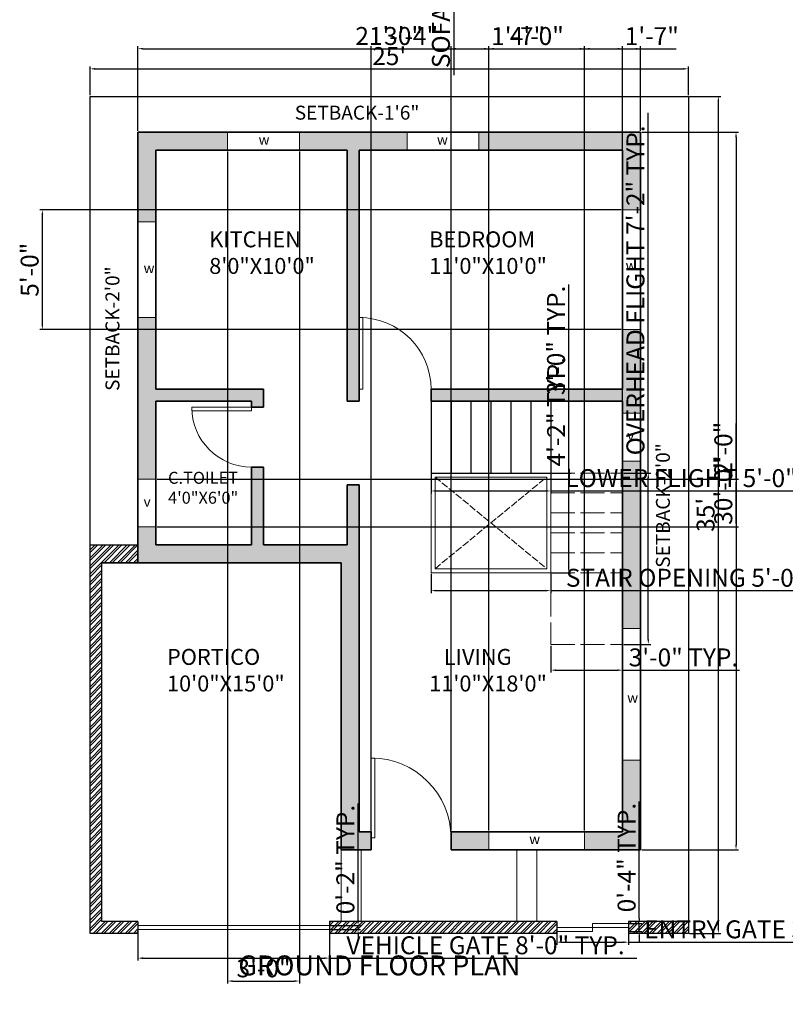
# Model space of a CAD drawing. Units: inches. Extents: x 3488 to 4319, y 780 to 1756.
# Tile 1 of 8: x 3488 to 3872, y 780 to 1274. Entities that reach past the tile are written whole.
import ezdxf

# ---------------------------------------------------------------- set-up
doc = ezdxf.new("R2010")
doc.units = ezdxf.units.IN
doc.linetypes.add('ACAD_ISO02W100', pattern=[15, 12, -3])
for name, color, linetype, lineweight in [('A-ANNO-IDEN', 7, 'Continuous', 13), ('A-ANNO-TEXT', 7, 'Continuous', 18), ('A-ANNO-TITL', 7, 'Continuous', 25), ('A-AREA-IDEN', 7, 'Continuous', 18), ('A-DOOR', 4, 'Continuous', 18), ('A-FLOR-OPEN', 3, 'Continuous', 20), ('A-FLOR-OPEN-HIDN', 3, 'ACAD_ISO02W100', 13), ('A-FLOR-OTLN', 7, 'Continuous', 20), ('A-FLOR-STRS', 7, 'Continuous', 25), ('A-FLOR-STRS-OVHD', 8, 'ACAD_ISO02W100', 18), ('A-WALL', 7, 'Continuous', 35), ('A-WALL-PATT', 252, 'Continuous', 13), ('C-PROP', 7, 'Continuous', 25), ('DIM', 9, 'Continuous', 18), ('L-FENC', 7, 'Continuous', 30), ('L-FENC-GATE', 4, 'Continuous', 18), ('L-FENC-PATT', 251, 'Continuous', 13), ('window', 130, 'Continuous', 18)]:
    doc.layers.add(name, color=color, linetype=linetype, lineweight=lineweight)
doc.styles.get("Standard").update_dxf_attribs({"font": 'arial.ttf'})
doc.dimstyles.new('ISO-25', dxfattribs={"dimtxt": 9, "dimasz": 2.5, "dimexe": 1.25, "dimexo": 0.625, "dimtad": 1, "dimdec": 1, "dimlunit": 3, "dimtxsty": 'Standard', "dimcen": 2.5, "dimclrd": 1, "dimclre": 1, "dimclrt": 1, "dimadec": 0, "dimazin": 0, "dimtfac": 1, "dimtdec": 1, "dimtmove": 0, "dimatfit": 3, "dimfxl": 1, "dimarcsym": 0})

# ---------------------------------------------------------------- blocks, each defined once
blk = doc.blocks.new('*U2')
for p, q in [((0, 0), (0, -6)), ((40, 0), (40, -6))]:
    blk.add_line(p, q)
blk.add_lwpolyline([(0, 0), (0, 40), (1.75, 40), (1.75, 0)], close=True)
blk.add_arc((0, 0), 40, 0, 90)
blk = doc.blocks.new('*U3')
for p, q in [((0, 0), (0, -6)), ((36, 0), (36, -6))]:
    blk.add_line(p, q)
blk.add_lwpolyline([(0, 0), (0, 36), (1.75, 36), (1.75, 0)], close=True)
blk.add_arc((0, 0), 36, 0, 90)
blk = doc.blocks.new('*U4')
for p, q in [((-30, 0), (-30, -6)), ((0, 0), (0, -6))]:
    blk.add_line(p, q)
blk.add_lwpolyline([(0, 0), (0, 30), (-1.75, 30), (-1.75, 0)], close=True)
blk.add_arc((0, 0), 30, 90, 180)
blk = doc.blocks.new('*D14')
at = {"layer": 'Defpoints', "color": 0, "transparency": 16777216}
for p in [(3822.99, 1249.81), (3522.99, 1236.01), (3822.99, 1236.01)]:
    blk.add_point(p, dxfattribs=at)
at = {"layer": 'DIM', "color": 0, "lineweight": -2, "transparency": 16777216}
for p, q in [((3522.99, 1236.63), (3522.99, 1251.06)), ((3822.99, 1236.63), (3822.99, 1251.06)), ((3525.49, 1249.81), (3820.49, 1249.81))]:
    blk.add_line(p, q, dxfattribs=at)
at = {"layer": 'DIM', "color": 0, "transparency": 16777216}
for points in [[(3525.49, 1250.23), (3525.49, 1249.39), (3522.99, 1249.81)], [(3820.49, 1250.23), (3820.49, 1249.39), (3822.99, 1249.81)]]:
    blk.add_solid(points, dxfattribs=at)
at = {"layer": 'DIM', "color": 0, "transparency": 16777216, "insert": (3672.99, 1255.03), "char_height": 9, "attachment_point": 5}
blk.add_mtext("25'", dxfattribs=at)
blk = doc.blocks.new('*D15')
at = {"layer": 'Defpoints', "color": 0, "transparency": 16777216}
for p in [(3822.99, 1236.01), (3822.99, 816.01), (3838.01, 816.01)]:
    blk.add_point(p, dxfattribs=at)
at = {"layer": 'DIM', "color": 0, "lineweight": -2, "transparency": 16777216}
for p, q in [((3823.61, 1236.01), (3839.26, 1236.01)), ((3838.01, 1233.51), (3838.01, 818.51)), ((3823.61, 816.01), (3839.26, 816.01))]:
    blk.add_line(p, q, dxfattribs=at)
at = {"layer": 'DIM', "color": 0, "transparency": 16777216}
for points in [[(3837.59, 1233.51), (3838.43, 1233.51), (3838.01, 1236.01)], [(3837.59, 818.51), (3838.43, 818.51), (3838.01, 816.01)]]:
    blk.add_solid(points, dxfattribs=at)
at = {"layer": 'DIM', "color": 0, "transparency": 16777216, "insert": (3832.79, 1026.01), "char_height": 9, "attachment_point": 5, "rotation": 90}
blk.add_mtext("35'", dxfattribs=at)
blk = doc.blocks.new('GATE-VEHICLE-96IN')
for p, q in [((0, 2), (96, 2)), ((0, 0), (96, 0))]:
    blk.add_line(p, q)
blk = doc.blocks.new('GATE-PEDESTRIAN-36IN')
for p, q in [((0, 2), (36, 2)), ((0, 0), (18, 0)), ((18, 4), (36, 4)), ((18, 4), (18, 0))]:
    blk.add_line(p, q)
blk = doc.blocks.new('STAIR-GROUND-LOWER-FLIGHT')
for p, q in [((0, 36), (0, 0)), ((10, 36), (10, 0)), ((20, 36), (20, 0)), ((30, 36), (30, 0)), ((40, 36), (40, 0)), ((50, 36), (50, 0)), ((60, 36), (60, 0)), ((0, 0), (60, 0))]:
    blk.add_line(p, q)
blk = doc.blocks.new('STAIR-GROUND-OVERHEAD-FLIGHT')
for p, q in [((0, 86), (0, 0)), ((0, 86), (36, 86)), ((0, 76), (36, 76)), ((0, 66), (36, 66)), ((0, 56), (36, 56)), ((0, 46), (36, 46)), ((0, 36), (36, 36)), ((0, 0), (36, 0))]:
    blk.add_line(p, q)
blk = doc.blocks.new('OPENING-STAIRWELL-FRAME')
for points in [[(60, 50), (0, 50), (0, 0), (60, 0)], [(58, 48), (2, 48), (2, 2), (58, 2)]]:
    blk.add_lwpolyline(points, close=True)
blk = doc.blocks.new('*D60')
at = {"layer": 'Defpoints', "color": 0, "transparency": 16777216}
for p in [(3693.99, 997.01), (3753.99, 997.01), (3753.99, 988.01)]:
    blk.add_point(p, dxfattribs=at)
at = {"layer": 'DIM', "color": 1, "lineweight": -2, "transparency": 16777216}
for p, q in [((3693.99, 996.38), (3693.99, 986.76)), ((3753.99, 996.38), (3753.99, 986.76)), ((3696.49, 988.01), (3751.49, 988.01)), ((3753.99, 988.01), (3914.55, 988.01))]:
    blk.add_line(p, q, dxfattribs=at)
at = {"layer": 'DIM', "color": 1, "transparency": 16777216}
for points in [[(3696.49, 988.42), (3696.49, 987.59), (3693.99, 988.01)], [(3751.49, 988.42), (3751.49, 987.59), (3753.99, 988.01)]]:
    blk.add_solid(points, dxfattribs=at)
at = {"layer": 'DIM', "color": 1, "transparency": 16777216, "insert": (3835.52, 993.29), "char_height": 9, "attachment_point": 5}
blk.add_mtext('STAIR OPENING 5\'-0" TYP.', dxfattribs=at)
blk = doc.blocks.new('*D61')
at = {"layer": 'Defpoints', "color": 0, "transparency": 16777216}
for p in [(3753.99, 1047.01), (3762.99, 1047.01), (3753.99, 997.01)]:
    blk.add_point(p, dxfattribs=at)
at = {"layer": 'DIM', "color": 1, "lineweight": -2, "transparency": 16777216}
for p, q in [((3762.99, 1047.01), (3762.99, 1105.98)), ((3754.61, 1047.01), (3764.24, 1047.01)), ((3762.99, 999.51), (3762.99, 1044.51)), ((3754.61, 997.01), (3764.24, 997.01))]:
    blk.add_line(p, q, dxfattribs=at)
at = {"layer": 'DIM', "color": 1, "transparency": 16777216}
for points in [[(3762.57, 1044.51), (3763.41, 1044.51), (3762.99, 1047.01)], [(3762.57, 999.51), (3763.41, 999.51), (3762.99, 997.01)]]:
    blk.add_solid(points, dxfattribs=at)
at = {"layer": 'DIM', "color": 1, "transparency": 16777216, "insert": (3757.84, 1077.74), "char_height": 9, "attachment_point": 5, "rotation": 90}
blk.add_mtext('4\'-2" TYP.', dxfattribs=at)
blk = doc.blocks.new('*D68')
at = {"layer": 'Defpoints', "color": 0, "transparency": 16777216}
for p in [(3546.99, 818.01), (3642.99, 818.01), (3642.99, 803.61)]:
    blk.add_point(p, dxfattribs=at)
at = {"layer": 'DIM', "color": 1, "lineweight": -2, "transparency": 16777216}
for p, q in [((3546.99, 817.38), (3546.99, 802.36)), ((3642.99, 817.38), (3642.99, 802.36)), ((3549.49, 803.61), (3640.49, 803.61)), ((3642.99, 803.61), (3797.09, 803.61))]:
    blk.add_line(p, q, dxfattribs=at)
at = {"layer": 'DIM', "color": 1, "transparency": 16777216}
for points in [[(3549.49, 804.02), (3549.49, 803.19), (3546.99, 803.61)], [(3640.49, 804.02), (3640.49, 803.19), (3642.99, 803.61)]]:
    blk.add_solid(points, dxfattribs=at)
at = {"layer": 'DIM', "color": 1, "transparency": 16777216, "insert": (3721.29, 808.89), "char_height": 9, "attachment_point": 5}
blk.add_mtext('VEHICLE GATE 8\'-0" TYP.', dxfattribs=at)
blk = doc.blocks.new('*D69')
at = {"layer": 'Defpoints', "color": 0, "transparency": 16777216}
for p in [(3642.99, 820.01), (3642.99, 818.01), (3657.39, 820.01)]:
    blk.add_point(p, dxfattribs=at)
at = {"layer": 'DIM', "color": 1, "lineweight": -2, "transparency": 16777216}
for p, q in [((3657.39, 822.51), (3657.39, 881.12)), ((3643.61, 820.01), (3658.64, 820.01)), ((3643.61, 818.01), (3658.64, 818.01)), ((3657.39, 818.01), (3657.39, 820.01)), ((3657.39, 815.51), (3657.39, 813.01))]:
    blk.add_line(p, q, dxfattribs=at)
at = {"layer": 'DIM', "color": 1, "transparency": 16777216}
for points in [[(3656.97, 822.51), (3657.81, 822.51), (3657.39, 820.01)], [(3656.97, 815.51), (3657.81, 815.51), (3657.39, 818.01)]]:
    blk.add_solid(points, dxfattribs=at)
at = {"layer": 'DIM', "color": 1, "transparency": 16777216, "insert": (3652.17, 853.06), "char_height": 9, "attachment_point": 5, "rotation": 90}
blk.add_mtext('0\'-2" TYP.', dxfattribs=at)
blk = doc.blocks.new('*D70')
at = {"layer": 'Defpoints', "color": 0, "transparency": 16777216}
for p in [(3756.99, 817.01), (3792.99, 817.01), (3792.99, 811.61)]:
    blk.add_point(p, dxfattribs=at)
at = {"layer": 'DIM', "color": 1, "lineweight": -2, "transparency": 16777216}
for p, q in [((3756.99, 816.38), (3756.99, 810.36)), ((3792.99, 816.38), (3792.99, 810.36)), ((3759.49, 811.61), (3790.49, 811.61)), ((3792.99, 811.61), (3934.96, 811.61))]:
    blk.add_line(p, q, dxfattribs=at)
at = {"layer": 'DIM', "color": 1, "transparency": 16777216}
for points in [[(3759.49, 812.02), (3759.49, 811.19), (3756.99, 811.61)], [(3790.49, 812.02), (3790.49, 811.19), (3792.99, 811.61)]]:
    blk.add_solid(points, dxfattribs=at)
at = {"layer": 'DIM', "color": 1, "transparency": 16777216, "insert": (3865.22, 816.89), "char_height": 9, "attachment_point": 5}
blk.add_mtext('ENTRY GATE 3\'-0" TYP.', dxfattribs=at)
blk = doc.blocks.new('*D71')
at = {"layer": 'Defpoints', "color": 0, "transparency": 16777216}
for p in [(3792.99, 821.01), (3798.39, 821.01), (3792.99, 817.01)]:
    blk.add_point(p, dxfattribs=at)
at = {"layer": 'DIM', "color": 1, "lineweight": -2, "transparency": 16777216}
for p, q in [((3798.39, 823.51), (3798.39, 882.12)), ((3793.61, 821.01), (3799.64, 821.01)), ((3798.39, 817.01), (3798.39, 821.01)), ((3793.61, 817.01), (3799.64, 817.01)), ((3798.39, 814.51), (3798.39, 812.01))]:
    blk.add_line(p, q, dxfattribs=at)
at = {"layer": 'DIM', "color": 1, "transparency": 16777216}
for points in [[(3797.97, 823.51), (3798.81, 823.51), (3798.39, 821.01)], [(3797.97, 814.51), (3798.81, 814.51), (3798.39, 817.01)]]:
    blk.add_solid(points, dxfattribs=at)
at = {"layer": 'DIM', "color": 1, "transparency": 16777216, "insert": (3793.17, 854.06), "char_height": 9, "attachment_point": 5, "rotation": 90}
blk.add_mtext('0\'-4" TYP.', dxfattribs=at)
blk = doc.blocks.new('*D74')
at = {"layer": 'Defpoints', "color": 0, "transparency": 16777216}
for p in [(3693.99, 1047.01), (3753.99, 1047.01), (3753.99, 1038.01)]:
    blk.add_point(p, dxfattribs=at)
at = {"layer": 'DIM', "color": 1, "lineweight": -2, "transparency": 16777216}
for p, q in [((3693.99, 1046.38), (3693.99, 1036.76)), ((3753.99, 1046.38), (3753.99, 1036.76)), ((3696.49, 1038.01), (3751.49, 1038.01)), ((3753.99, 1038.01), (3910, 1038.01))]:
    blk.add_line(p, q, dxfattribs=at)
at = {"layer": 'DIM', "color": 1, "transparency": 16777216}
for points in [[(3696.49, 1038.42), (3696.49, 1037.59), (3693.99, 1038.01)], [(3751.49, 1038.42), (3751.49, 1037.59), (3753.99, 1038.01)]]:
    blk.add_solid(points, dxfattribs=at)
at = {"layer": 'DIM', "color": 1, "transparency": 16777216, "insert": (3833.24, 1043.29), "char_height": 9, "attachment_point": 5}
blk.add_mtext('LOWER FLIGHT 5\'-0" TYP.', dxfattribs=at)
blk = doc.blocks.new('*D75')
at = {"layer": 'Defpoints', "color": 0, "transparency": 16777216}
for p in [(3753.99, 1083.01), (3762.99, 1083.01), (3753.99, 1047.01)]:
    blk.add_point(p, dxfattribs=at)
at = {"layer": 'DIM', "color": 1, "lineweight": -2, "transparency": 16777216}
for p, q in [((3762.99, 1083.01), (3762.99, 1141.61)), ((3754.61, 1083.01), (3764.24, 1083.01)), ((3762.99, 1049.51), (3762.99, 1080.51)), ((3754.61, 1047.01), (3764.24, 1047.01))]:
    blk.add_line(p, q, dxfattribs=at)
at = {"layer": 'DIM', "color": 1, "transparency": 16777216}
for points in [[(3762.57, 1080.51), (3763.41, 1080.51), (3762.99, 1083.01)], [(3762.57, 1049.51), (3763.41, 1049.51), (3762.99, 1047.01)]]:
    blk.add_solid(points, dxfattribs=at)
at = {"layer": 'DIM', "color": 1, "transparency": 16777216, "insert": (3757.77, 1113.56), "char_height": 9, "attachment_point": 5, "rotation": 90}
blk.add_mtext('3\'-0" TYP.', dxfattribs=at)
blk = doc.blocks.new('*D76')
at = {"layer": 'Defpoints', "color": 0, "transparency": 16777216}
for p in [(3789.99, 1047.01), (3802.89, 1047.01), (3789.99, 961.01)]:
    blk.add_point(p, dxfattribs=at)
at = {"layer": 'DIM', "color": 1, "lineweight": -2, "transparency": 16777216}
for p, q in [((3802.89, 1047.01), (3802.89, 1227.79)), ((3790.61, 1047.01), (3804.14, 1047.01)), ((3802.89, 963.51), (3802.89, 1044.51)), ((3790.61, 961.01), (3804.14, 961.01))]:
    blk.add_line(p, q, dxfattribs=at)
at = {"layer": 'DIM', "color": 1, "transparency": 16777216}
for points in [[(3802.47, 1044.51), (3803.31, 1044.51), (3802.89, 1047.01)], [(3802.47, 963.51), (3803.31, 963.51), (3802.89, 961.01)]]:
    blk.add_solid(points, dxfattribs=at)
at = {"layer": 'DIM', "color": 1, "transparency": 16777216, "insert": (3797.61, 1138.65), "char_height": 9, "attachment_point": 5, "rotation": 90}
blk.add_mtext('OVERHEAD FLIGHT 7\'-2" TYP.', dxfattribs=at)
blk = doc.blocks.new('*D77')
at = {"layer": 'Defpoints', "color": 0, "transparency": 16777216}
for p in [(3753.99, 961.01), (3789.99, 961.01), (3789.99, 948.11)]:
    blk.add_point(p, dxfattribs=at)
at = {"layer": 'DIM', "color": 1, "lineweight": -2, "transparency": 16777216}
for p, q in [((3753.99, 960.38), (3753.99, 946.86)), ((3789.99, 960.38), (3789.99, 946.86)), ((3756.49, 948.11), (3787.49, 948.11)), ((3789.99, 948.11), (3848.59, 948.11))]:
    blk.add_line(p, q, dxfattribs=at)
at = {"layer": 'DIM', "color": 1, "transparency": 16777216}
for points in [[(3756.49, 948.52), (3756.49, 947.69), (3753.99, 948.11)], [(3787.49, 948.52), (3787.49, 947.69), (3789.99, 948.11)]]:
    blk.add_solid(points, dxfattribs=at)
at = {"layer": 'DIM', "color": 1, "transparency": 16777216, "insert": (3820.54, 953.33), "char_height": 9, "attachment_point": 5}
blk.add_mtext('3\'-0" TYP.', dxfattribs=at)
blk = doc.blocks.new('*D102')
at = {"layer": 'Defpoints', "color": 0, "transparency": 16777216}
for p in [(3719, 1452.36), (3705.37, 1361.55), (3719, 1361.55)]:
    blk.add_point(p, dxfattribs=at)
at = {"layer": 'DIM', "color": 1, "lineweight": -2, "transparency": 16777216}
for p, q in [((3718.37, 1452.36), (3704.12, 1452.36)), ((3705.37, 1449.86), (3705.37, 1364.05)), ((3718.37, 1361.55), (3704.12, 1361.55)), ((3705.37, 1361.55), (3705.37, 1246.6))]:
    blk.add_line(p, q, dxfattribs=at)
at = {"layer": 'DIM', "color": 1, "transparency": 16777216}
for points in [[(3704.96, 1449.86), (3705.79, 1449.86), (3705.37, 1452.36)], [(3704.96, 1364.05), (3705.79, 1364.05), (3705.37, 1361.55)]]:
    blk.add_solid(points, dxfattribs=at)
at = {"layer": 'DIM', "color": 1, "transparency": 16777216, "insert": (3700.09, 1302.83), "char_height": 9, "attachment_point": 5, "rotation": 90}
blk.add_mtext('SOFA GROUP 7\'-7"', dxfattribs=at)
blk = doc.blocks.new('*D108')
at = {"layer": 'Defpoints', "color": 0, "transparency": 16777216}
for p in [(3798.99, 1259.91), (3546.99, 1218.01), (3798.99, 1218.01)]:
    blk.add_point(p, dxfattribs=at)
at = {"layer": 'DIM', "color": 1, "lineweight": -2, "transparency": 16777216}
for p, q in [((3546.99, 1218.63), (3546.99, 1261.16)), ((3549.49, 1259.91), (3796.49, 1259.91)), ((3798.99, 1218.63), (3798.99, 1261.16))]:
    blk.add_line(p, q, dxfattribs=at)
at = {"layer": 'DIM', "color": 1, "transparency": 16777216}
for points in [[(3549.49, 1260.32), (3549.49, 1259.49), (3546.99, 1259.91)], [(3796.49, 1260.32), (3796.49, 1259.49), (3798.99, 1259.91)]]:
    blk.add_solid(points, dxfattribs=at)
at = {"layer": 'DIM', "color": 1, "transparency": 16777216, "insert": (3672.99, 1265.13), "char_height": 9, "attachment_point": 5}
blk.add_mtext('21\'-0"', dxfattribs=at)
blk = doc.blocks.new('*D109')
at = {"layer": 'Defpoints', "color": 0, "transparency": 16777216}
for p in [(3798.99, 1218.01), (3798.99, 858.01), (3846.89, 858.01)]:
    blk.add_point(p, dxfattribs=at)
at = {"layer": 'DIM', "color": 1, "lineweight": -2, "transparency": 16777216}
for p, q in [((3799.61, 1218.01), (3848.14, 1218.01)), ((3846.89, 1215.51), (3846.89, 860.51)), ((3799.61, 858.01), (3848.14, 858.01))]:
    blk.add_line(p, q, dxfattribs=at)
at = {"layer": 'DIM', "color": 1, "transparency": 16777216}
for points in [[(3846.47, 1215.51), (3847.31, 1215.51), (3846.89, 1218.01)], [(3846.47, 860.51), (3847.31, 860.51), (3846.89, 858.01)]]:
    blk.add_solid(points, dxfattribs=at)
at = {"layer": 'DIM', "color": 1, "transparency": 16777216, "insert": (3841.67, 1038.01), "char_height": 9, "attachment_point": 5, "rotation": 90}
blk.add_mtext('30\'-0"', dxfattribs=at)
blk = doc.blocks.new('*D112')
at = {"layer": 'Defpoints', "color": 0, "transparency": 16777216}
for p in [(3703.99, 1259.91), (3663.99, 867.01), (3703.99, 867.01)]:
    blk.add_point(p, dxfattribs=at)
at = {"layer": 'DIM', "color": 1, "lineweight": -2, "transparency": 16777216}
for p, q in [((3663.99, 867.63), (3663.99, 1261.16)), ((3666.49, 1259.91), (3701.49, 1259.91)), ((3703.99, 867.63), (3703.99, 1261.16))]:
    blk.add_line(p, q, dxfattribs=at)
at = {"layer": 'DIM', "color": 1, "transparency": 16777216}
for points in [[(3666.49, 1260.32), (3666.49, 1259.49), (3663.99, 1259.91)], [(3701.49, 1260.32), (3701.49, 1259.49), (3703.99, 1259.91)]]:
    blk.add_solid(points, dxfattribs=at)
at = {"layer": 'DIM', "color": 1, "transparency": 16777216, "insert": (3683.99, 1265.13), "char_height": 9, "attachment_point": 5}
blk.add_mtext('3\'-4"', dxfattribs=at)
blk = doc.blocks.new('*D113')
at = {"layer": 'Defpoints', "color": 0, "transparency": 16777216}
for p in [(3722.99, 1259.91), (3703.99, 867.01), (3722.99, 867.01)]:
    blk.add_point(p, dxfattribs=at)
at = {"layer": 'DIM', "color": 1, "lineweight": -2, "transparency": 16777216}
for p, q in [((3703.99, 867.63), (3703.99, 1261.16)), ((3706.49, 1259.91), (3720.49, 1259.91)), ((3722.99, 867.63), (3722.99, 1261.16)), ((3722.99, 1259.91), (3749.82, 1259.91))]:
    blk.add_line(p, q, dxfattribs=at)
at = {"layer": 'DIM', "color": 1, "transparency": 16777216}
for points in [[(3706.49, 1260.32), (3706.49, 1259.49), (3703.99, 1259.91)], [(3720.49, 1260.32), (3720.49, 1259.49), (3722.99, 1259.91)]]:
    blk.add_solid(points, dxfattribs=at)
at = {"layer": 'DIM', "color": 1, "transparency": 16777216, "insert": (3737.65, 1265.05), "char_height": 9, "attachment_point": 5}
blk.add_mtext('1\'-7"', dxfattribs=at)
blk = doc.blocks.new('*D114')
at = {"layer": 'Defpoints', "color": 0, "transparency": 16777216}
for p in [(3770.99, 1259.91), (3722.99, 867.01), (3770.99, 867.01)]:
    blk.add_point(p, dxfattribs=at)
at = {"layer": 'DIM', "color": 1, "lineweight": -2, "transparency": 16777216}
for p, q in [((3722.99, 867.63), (3722.99, 1261.16)), ((3725.49, 1259.91), (3768.49, 1259.91)), ((3770.99, 867.63), (3770.99, 1261.16))]:
    blk.add_line(p, q, dxfattribs=at)
at = {"layer": 'DIM', "color": 1, "transparency": 16777216}
for points in [[(3725.49, 1260.32), (3725.49, 1259.49), (3722.99, 1259.91)], [(3768.49, 1260.32), (3768.49, 1259.49), (3770.99, 1259.91)]]:
    blk.add_solid(points, dxfattribs=at)
at = {"layer": 'DIM', "color": 1, "transparency": 16777216, "insert": (3746.99, 1265.13), "char_height": 9, "attachment_point": 5}
blk.add_mtext('4\'-0"', dxfattribs=at)
blk = doc.blocks.new('*D115')
at = {"layer": 'Defpoints', "color": 0, "transparency": 16777216}
for p in [(3789.99, 1259.91), (3770.99, 867.01), (3789.99, 867.01)]:
    blk.add_point(p, dxfattribs=at)
at = {"layer": 'DIM', "color": 1, "lineweight": -2, "transparency": 16777216}
for p, q in [((3770.99, 867.63), (3770.99, 1261.16)), ((3773.49, 1259.91), (3787.49, 1259.91)), ((3789.99, 867.63), (3789.99, 1261.16)), ((3789.99, 1259.91), (3816.82, 1259.91))]:
    blk.add_line(p, q, dxfattribs=at)
at = {"layer": 'DIM', "color": 1, "transparency": 16777216}
for points in [[(3773.49, 1260.32), (3773.49, 1259.49), (3770.99, 1259.91)], [(3787.49, 1260.32), (3787.49, 1259.49), (3789.99, 1259.91)]]:
    blk.add_solid(points, dxfattribs=at)
at = {"layer": 'DIM', "color": 1, "transparency": 16777216, "insert": (3804.65, 1265.05), "char_height": 9, "attachment_point": 5}
blk.add_mtext('1\'-7"', dxfattribs=at)
blk = doc.blocks.new('*D116')
at = {"layer": 'Defpoints', "color": 0, "transparency": 16777216}
for p in [(3591.99, 1209.01), (3627.99, 1209.01), (3627.99, 792.11)]:
    blk.add_point(p, dxfattribs=at)
at = {"layer": 'DIM', "color": 1, "lineweight": -2, "transparency": 16777216}
for p, q in [((3591.99, 1208.38), (3591.99, 790.86)), ((3627.99, 1208.38), (3627.99, 790.86)), ((3594.49, 792.11), (3625.49, 792.11))]:
    blk.add_line(p, q, dxfattribs=at)
at = {"layer": 'DIM', "color": 1, "transparency": 16777216}
for points in [[(3594.49, 792.52), (3594.49, 791.69), (3591.99, 792.11)], [(3625.49, 792.52), (3625.49, 791.69), (3627.99, 792.11)]]:
    blk.add_solid(points, dxfattribs=at)
at = {"layer": 'DIM', "color": 1, "transparency": 16777216, "insert": (3609.99, 797.33), "char_height": 9, "attachment_point": 5}
blk.add_mtext('3\'-0"', dxfattribs=at)
blk = doc.blocks.new('*D117')
at = {"layer": 'Defpoints', "color": 0, "transparency": 16777216}
for p in [(3499.09, 1179.01), (3789.99, 1179.01), (3789.99, 1119.01)]:
    blk.add_point(p, dxfattribs=at)
at = {"layer": 'DIM', "color": 1, "lineweight": -2, "transparency": 16777216}
for p, q in [((3789.36, 1179.01), (3497.84, 1179.01)), ((3499.09, 1121.51), (3499.09, 1176.51)), ((3789.36, 1119.01), (3497.84, 1119.01))]:
    blk.add_line(p, q, dxfattribs=at)
at = {"layer": 'DIM', "color": 1, "transparency": 16777216}
for points in [[(3498.67, 1176.51), (3499.51, 1176.51), (3499.09, 1179.01)], [(3498.67, 1121.51), (3499.51, 1121.51), (3499.09, 1119.01)]]:
    blk.add_solid(points, dxfattribs=at)
at = {"layer": 'DIM', "color": 1, "transparency": 16777216, "insert": (3493.87, 1149.01), "char_height": 9, "attachment_point": 5, "rotation": 90}
blk.add_mtext('5\'-0"', dxfattribs=at)
blk = doc.blocks.new('*D118')
at = {"layer": 'Defpoints', "color": 0, "transparency": 16777216}
for p in [(3555.99, 1044.01), (3846.89, 1044.01), (3555.99, 1020.01)]:
    blk.add_point(p, dxfattribs=at)
at = {"layer": 'DIM', "color": 1, "lineweight": -2, "transparency": 16777216}
for p, q in [((3846.89, 1044.01), (3846.89, 1071.84)), ((3556.61, 1044.01), (3848.14, 1044.01)), ((3846.89, 1022.51), (3846.89, 1041.51)), ((3556.61, 1020.01), (3848.14, 1020.01))]:
    blk.add_line(p, q, dxfattribs=at)
at = {"layer": 'DIM', "color": 1, "transparency": 16777216}
for points in [[(3846.47, 1041.51), (3847.31, 1041.51), (3846.89, 1044.01)], [(3846.47, 1022.51), (3847.31, 1022.51), (3846.89, 1020.01)]]:
    blk.add_solid(points, dxfattribs=at)
at = {"layer": 'DIM', "color": 1, "transparency": 16777216, "insert": (3841.67, 1059.17), "char_height": 9, "attachment_point": 5, "rotation": 90}
blk.add_mtext('2\'-0"', dxfattribs=at)

msp = doc.modelspace()

# ---------------------------------------------------------------- hatches: boundary and pattern name
at = {"layer": 'A-WALL-PATT'}
h = msp.add_hatch(color=256, dxfattribs=at)
h.dxf.hatch_style = 1
h.paths.add_polyline_path([(3546.99, 1218.01), (3546.99, 1173.01), (3555.99, 1173.01), (3555.99, 1209.01), (3591.99, 1209.01), (3591.99, 1218.01)])
h.paths.add_polyline_path([(3651.99, 1209.01), (3651.99, 1083.01), (3657.99, 1083.01), (3657.99, 1089.01), (3657.99, 1125.01), (3657.99, 1209.01), (3681.99, 1209.01), (3681.99, 1218.01), (3627.99, 1218.01), (3627.99, 1209.01)])
h.paths.add_polyline_path([(3789.99, 1209.01), (3789.99, 1179.01), (3798.99, 1179.01), (3798.99, 1218.01), (3717.99, 1218.01), (3717.99, 1209.01)])
h.paths.add_polyline_path([(3789.99, 1089.01), (3693.99, 1089.01), (3693.99, 1083.01), (3789.99, 1083.01), (3789.99, 1077.04), (3798.99, 1077.04), (3798.99, 1119.01), (3789.99, 1119.01)])
h.paths.add_polyline_path([(3546.99, 1044.01), (3555.99, 1044.01), (3555.99, 1083.01), (3603.99, 1083.01), (3603.99, 1080.01), (3609.99, 1080.01), (3609.99, 1089.01), (3555.99, 1089.01), (3555.99, 1125.01), (3546.99, 1125.01)])
h.paths.add_polyline_path([(3648.99, 1002.01), (3648.99, 858.01), (3663.99, 858.01), (3663.99, 867.01), (3657.99, 867.01), (3657.99, 1011.01), (3657.99, 1041.01), (3651.99, 1041.01), (3651.99, 1011.01), (3609.99, 1011.01), (3609.99, 1050.01), (3603.99, 1050.01), (3603.99, 1011.01), (3555.99, 1011.01), (3555.99, 1020.01), (3546.99, 1020.01), (3546.99, 1002.01)])
h.paths.add_polyline_path([(3703.99, 867.01), (3703.99, 858.01), (3722.99, 858.01), (3722.99, 867.01)])
h.paths.add_polyline_path([(3770.99, 867.01), (3770.99, 858.01), (3798.99, 858.01), (3798.99, 903.01), (3789.99, 903.01), (3789.99, 867.01)])
h.paths.add_polyline_path([(3798.99, 1053.04), (3789.99, 1053.04), (3789.99, 969.01), (3798.99, 969.01)])
at = {"layer": 'L-FENC-PATT'}
h = msp.add_hatch(dxfattribs=at)
h.set_pattern_fill('ANSI32', color=256, scale=0.3)
h.set_pattern_definition([(45, (0, -1100.1302), (-2.0205576, 2.0205576), []), (45, (1.347, -1100.1302), (-2.0205576, 2.0205576), [])])
h.paths.add_polyline_path([(3528.99, 1002.01), (3546.99, 1002.01), (3546.99, 1011.01), (3522.99, 1011.01), (3522.99, 816.01), (3546.99, 816.01), (3546.99, 822.01), (3528.99, 822.01)])
h.paths.add_polyline_path([(3642.99, 822.01), (3642.99, 816.01), (3756.99, 816.01), (3756.99, 822.01)])
h.paths.add_polyline_path([(3792.99, 822.01), (3792.99, 816.01), (3822.99, 816.01), (3822.99, 822.01)])

# ---------------------------------------------------------------- linework, layer by layer
at = {"layer": 'A-FLOR-OPEN-HIDN', "ltscale": 0.3}
for p, q in [((3695.99, 1045.01), (3751.99, 999.01)), ((3695.99, 999.01), (3751.99, 1045.01))]:
    msp.add_line(p, q, dxfattribs=at)
at = {"layer": 'A-FLOR-OTLN'}
for p, q in [((3648.99, 858.01), (3648.99, 822.01)), ((3658.99, 858.01), (3658.99, 822.01)), ((3736.99, 858.01), (3736.99, 822.01)), ((3746.99, 858.01), (3746.99, 822.01))]:
    msp.add_line(p, q, dxfattribs=at)
at = {"layer": 'A-WALL'}
for p, q in [((3546.99, 1218.01), (3798.99, 1218.01)), ((3546.99, 1002.01), (3546.99, 1218.01)), ((3798.99, 1218.01), (3798.99, 858.01)), ((3555.99, 1209.01), (3651.99, 1209.01)), ((3555.99, 1089.01), (3555.99, 1209.01)), ((3651.99, 1209.01), (3651.99, 1083.01)), ((3657.99, 1209.01), (3789.99, 1209.01)), ((3657.99, 1209.01), (3657.99, 1083.01)), ((3789.99, 1209.01), (3789.99, 1089.01)), ((3555.99, 1089.01), (3609.99, 1089.01)), ((3609.99, 1080.01), (3609.99, 1089.01)), ((3693.99, 1089.01), (3789.99, 1089.01)), ((3693.99, 1089.01), (3693.99, 1083.01)), ((3555.99, 1083.01), (3603.99, 1083.01)), ((3555.99, 1011.01), (3555.99, 1083.01)), ((3603.99, 1080.01), (3603.99, 1083.01)), ((3651.99, 1083.01), (3657.99, 1083.01)), ((3693.99, 1083.01), (3789.99, 1083.01)), ((3789.99, 1083.01), (3789.99, 867.01)), ((3603.99, 1080.01), (3609.99, 1080.01)), ((3603.99, 1050.01), (3609.99, 1050.01)), ((3603.99, 1011.01), (3603.99, 1050.01)), ((3609.99, 1011.01), (3609.99, 1050.01)), ((3651.99, 1041.01), (3657.99, 1041.01)), ((3651.99, 1041.01), (3651.99, 1011.01)), ((3657.99, 1041.01), (3657.99, 1011.01)), ((3555.99, 1011.01), (3603.99, 1011.01)), ((3609.99, 1011.01), (3651.99, 1011.01)), ((3657.99, 1011.01), (3657.99, 867.01)), ((3528.99, 1002.01), (3648.99, 1002.01)), ((3648.99, 1002.01), (3648.99, 858.01)), ((3657.99, 867.01), (3663.99, 867.01)), ((3663.99, 867.01), (3663.99, 858.01)), ((3703.99, 867.01), (3789.99, 867.01)), ((3703.99, 867.01), (3703.99, 858.01)), ((3648.99, 858.01), (3663.99, 858.01)), ((3703.99, 858.01), (3798.99, 858.01))]:
    msp.add_line(p, q, dxfattribs=at)
at = {"layer": 'C-PROP'}
for p, q in [((3522.99, 1236.01), (3822.99, 1236.01)), ((3522.99, 816.01), (3522.99, 1236.01)), ((3822.99, 1236.01), (3822.99, 816.01))]:
    msp.add_line(p, q, dxfattribs=at)
at = {"layer": 'L-FENC'}
for p, q in [((3522.99, 1011.01), (3546.99, 1011.01)), ((3528.99, 822.01), (3528.99, 1002.01)), ((3546.99, 822.01), (3528.99, 822.01)), ((3546.99, 822.01), (3546.99, 816.01)), ((3756.99, 822.01), (3642.99, 822.01)), ((3642.99, 822.01), (3642.99, 816.01)), ((3756.99, 822.01), (3756.99, 816.01)), ((3792.99, 822.01), (3792.99, 816.01)), ((3822.99, 822.01), (3792.99, 822.01)), ((3546.99, 816.01), (3522.99, 816.01)), ((3756.99, 816.01), (3642.99, 816.01)), ((3822.99, 816.01), (3792.99, 816.01))]:
    msp.add_line(p, q, dxfattribs=at)
at = {"layer": 'window'}
for p, q in [((3591.99, 1209.01), (3591.99, 1218.01)), ((3627.99, 1209.01), (3627.99, 1218.01)), ((3681.99, 1209.01), (3681.99, 1218.01)), ((3717.99, 1209.01), (3717.99, 1218.01)), ((3789.99, 1179.01), (3798.99, 1179.01)), ((3555.99, 1173.01), (3546.99, 1173.01)), ((3555.99, 1125.01), (3546.99, 1125.01)), ((3789.99, 1119.01), (3798.99, 1119.01)), ((3789.99, 1077.04), (3798.99, 1077.04)), ((3789.99, 1053.04), (3798.99, 1053.04)), ((3546.99, 1044.01), (3555.99, 1044.01)), ((3546.99, 1020.01), (3555.99, 1020.01)), ((3789.99, 969.01), (3798.99, 969.01)), ((3789.99, 903.01), (3798.99, 903.01)), ((3722.99, 867.01), (3722.99, 858.01)), ((3770.99, 867.01), (3770.99, 858.01))]:
    msp.add_line(p, q, dxfattribs=at)

# ---------------------------------------------------------------- block references
at = {"layer": 'A-DOOR'}
for name, p in [('*U3', (3657.99, 1089.01)), ('*U2', (3663.99, 864.01))]:
    msp.add_blockref(name, p, dxfattribs=at)
at = {"layer": 'A-DOOR', "rotation": 90}
msp.add_blockref('*U4', (3603.99, 1080.01), dxfattribs=at)
at = {"layer": 'A-FLOR-OPEN'}
msp.add_blockref('OPENING-STAIRWELL-FRAME', (3693.99, 997.01), dxfattribs=at)
at = {"layer": 'A-FLOR-STRS'}
msp.add_blockref('STAIR-GROUND-LOWER-FLIGHT', (3693.99, 1047.01), dxfattribs=at)
at = {"layer": 'A-FLOR-STRS-OVHD'}
msp.add_blockref('STAIR-GROUND-OVERHEAD-FLIGHT', (3753.99, 961.01), dxfattribs=at)
at = {"layer": 'L-FENC-GATE'}
for name, p in [('GATE-PEDESTRIAN-36IN', (3756.99, 817.01)), ('GATE-VEHICLE-96IN', (3546.99, 818.01))]:
    msp.add_blockref(name, p, dxfattribs=at)

# ---------------------------------------------------------------- texts
at = {"layer": 'A-ANNO-IDEN'}
for s, p in [('w', (3607.51, 1211.76)), ('w', (3696.94, 1211.76)), ('w', (3791.51, 1148.73)), ('w', (3549.85, 1147.3)), ('v', (3792.33, 1063.32)), ('v', (3549.85, 1030.1)), ('w', (3792.33, 931.74)), ('w', (3743.2, 860.84))]:
    msp.add_text(s, height=5, dxfattribs=at).set_placement(p)
at = {"layer": 'A-ANNO-TEXT', "insert": (3625.66, 1231.32), "char_height": 7, "attachment_point": 1}
msp.add_mtext_dynamic_manual_height_columns('\\pxt7;{SETBACK-1\'6"}', width=83.4163, gutter_width=25, heights=[0], dxfattribs=at)
at = {"layer": 'A-ANNO-TEXT', "char_height": 7, "attachment_point": 1, "rotation": 90}
for insert in [(3530.74, 1088.23), (3806.74, 999.48)]:
    msp.add_mtext_dynamic_manual_height_columns('\\pxt7;{SETBACK-2\'0"}', width=83.4163, gutter_width=25, heights=[0], dxfattribs=dict(at, insert=insert))
at = {"layer": 'A-ANNO-TITL', "insert": (3597.32, 804.94), "char_height": 10, "attachment_point": 1}
msp.add_mtext_dynamic_manual_height_columns('GROUND FLOOR PLAN', width=202.5735, gutter_width=25, heights=[0], dxfattribs=at)
at = {"layer": 'A-AREA-IDEN', "attachment_point": 1}
for s, insert, char_height in [('KITCHEN\\P8\'0"X10\'0"', (3582.75, 1168.26), 8), ('BEDROOM\\P11\'0"X10\'0"', (3693.04, 1168.26), 8), ('C.TOILET\\P4\'0"X6\'0"', (3562.14, 1047.61), 6), ('PORTICO\\P10\'0"X15\'0"', (3561.58, 958.74), 8), ('   LIVING\\P11\'0"X18\'0"', (3693.04, 958.74), 8)]:
    msp.add_mtext_dynamic_manual_height_columns(s, width=83.4163, gutter_width=25, heights=[0], dxfattribs=dict(at, insert=insert, char_height=char_height))

# ---------------------------------------------------------------- dimensions: what is measured, and where the dimension line sits
at = {"layer": 'DIM'}
for base, p1, p2, angle, text, picture, middle in [((3705.37, 1361.55), (3719, 1452.36), (3719, 1361.55), 270, 'SOFA GROUP <>', '*D102', (3700.09, 1302.83)), ((3802.89, 1047.01), (3789.99, 961.01), (3789.99, 1047.01), 90, 'OVERHEAD FLIGHT <> TYP.', '*D76', (3797.61, 1138.65)), ((3762.99, 1083.01), (3753.99, 1047.01), (3753.99, 1083.01), 90, '<> TYP.', '*D75', (3757.77, 1113.56)), ((3762.99, 1047.01), (3753.99, 997.01), (3753.99, 1047.01), 90, '<> TYP.', '*D61', (3757.84, 1077.74)), ((3657.39, 820.01), (3642.99, 818.01), (3642.99, 820.01), 90, '<> TYP.', '*D69', (3652.17, 853.06)), ((3798.39, 821.01), (3792.99, 817.01), (3792.99, 821.01), 90, '<> TYP.', '*D71', (3793.17, 854.06))]:
    dim = msp.add_linear_dim(base=base, p1=p1, p2=p2, angle=angle, text=text, dimstyle='ISO-25', override={"dimdec": 1, "dimlfac": 1, "dimrnd": 0, "dimzin": 1, "dimdsep": 46, "dimlunit": 4, "dimfrac": 2}, dxfattribs=at)
    dim.commit()
    dim.dimension.update_dxf_attribs({"geometry": picture, "text_midpoint": middle})
for base, p1, p2, override, picture, middle in [((3798.99, 1259.91), (3546.99, 1218.01), (3798.99, 1218.01), {"dimdec": 1, "dimlfac": 1, "dimrnd": 0, "dimzin": 1, "dimdsep": 46, "dimlunit": 4, "dimfrac": 2}, '*D108', (3672.99, 1265.13)), ((3703.99, 1259.91), (3663.99, 867.01), (3703.99, 867.01), {"dimdec": 1, "dimlfac": 1, "dimrnd": 0, "dimzin": 1, "dimdsep": 46, "dimlunit": 4, "dimfrac": 2}, '*D112', (3683.99, 1265.13)), ((3722.99, 1259.91), (3703.99, 867.01), (3722.99, 867.01), {"dimdec": 1, "dimlfac": 1, "dimrnd": 0, "dimzin": 1, "dimdsep": 46, "dimlunit": 4, "dimfrac": 2}, '*D113', (3737.65, 1265.05)), ((3770.99, 1259.91), (3722.99, 867.01), (3770.99, 867.01), {"dimdec": 1, "dimlfac": 1, "dimrnd": 0, "dimzin": 1, "dimdsep": 46, "dimlunit": 4, "dimfrac": 2}, '*D114', (3746.99, 1265.13)), ((3789.99, 1259.91), (3770.99, 867.01), (3789.99, 867.01), {"dimdec": 1, "dimlfac": 1, "dimrnd": 0, "dimzin": 1, "dimdsep": 46, "dimlunit": 4, "dimfrac": 2}, '*D115', (3804.65, 1265.05)), ((3822.99, 1249.81), (3522.99, 1236.01), (3822.99, 1236.01), {"dimclrd": 0, "dimclre": 0, "dimclrt": 0}, '*D14', (3672.99, 1255.03)), ((3627.99, 792.11), (3591.99, 1209.01), (3627.99, 1209.01), {"dimdec": 1, "dimlfac": 1, "dimrnd": 0, "dimzin": 1, "dimdsep": 46, "dimlunit": 4, "dimfrac": 2}, '*D116', (3609.99, 797.33))]:
    dim = msp.add_linear_dim(base=base, p1=p1, p2=p2, dimstyle='ISO-25', override=override, dxfattribs=at)
    dim.commit()
    dim.dimension.update_dxf_attribs({"geometry": picture, "text_midpoint": middle})
for base, p1, p2, override, picture, middle in [((3838.01, 816.01), (3822.99, 1236.01), (3822.99, 816.01), {"dimclrd": 0, "dimclre": 0, "dimclrt": 0}, '*D15', (3832.79, 1026.01)), ((3846.89, 858.01), (3798.99, 1218.01), (3798.99, 858.01), {"dimdec": 1, "dimlfac": 1, "dimrnd": 0, "dimzin": 1, "dimdsep": 46, "dimlunit": 4, "dimfrac": 2}, '*D109', (3841.67, 1038.01)), ((3499.09, 1179.01), (3789.99, 1119.01), (3789.99, 1179.01), {"dimdec": 1, "dimlfac": 1, "dimrnd": 0, "dimzin": 1, "dimdsep": 46, "dimlunit": 4, "dimfrac": 2}, '*D117', (3493.87, 1149.01)), ((3846.89, 1044.01), (3555.99, 1020.01), (3555.99, 1044.01), {"dimdec": 1, "dimlfac": 1, "dimrnd": 0, "dimzin": 1, "dimdsep": 46, "dimlunit": 4, "dimfrac": 2}, '*D118', (3841.67, 1059.17))]:
    dim = msp.add_linear_dim(base=base, p1=p1, p2=p2, angle=90, dimstyle='ISO-25', override=override, dxfattribs=at)
    dim.commit()
    dim.dimension.update_dxf_attribs({"geometry": picture, "text_midpoint": middle})
for base, p1, p2, text, picture, middle in [((3753.99, 1038.01), (3693.99, 1047.01), (3753.99, 1047.01), 'LOWER FLIGHT <> TYP.', '*D74', (3833.24, 1043.29)), ((3753.99, 988.01), (3693.99, 997.01), (3753.99, 997.01), 'STAIR OPENING <> TYP.', '*D60', (3835.52, 993.29)), ((3789.99, 948.11), (3753.99, 961.01), (3789.99, 961.01), '<> TYP.', '*D77', (3820.54, 953.33)), ((3792.99, 811.61), (3756.99, 817.01), (3792.99, 817.01), 'ENTRY GATE <> TYP.', '*D70', (3865.22, 816.89)), ((3642.99, 803.61), (3546.99, 818.01), (3642.99, 818.01), 'VEHICLE GATE <> TYP.', '*D68', (3721.29, 808.89))]:
    dim = msp.add_linear_dim(base=base, p1=p1, p2=p2, text=text, dimstyle='ISO-25', override={"dimdec": 1, "dimlfac": 1, "dimrnd": 0, "dimzin": 1, "dimdsep": 46, "dimlunit": 4, "dimfrac": 2}, dxfattribs=at)
    dim.commit()
    dim.dimension.update_dxf_attribs({"geometry": picture, "text_midpoint": middle})

doc.saveas('drawing.dxf')
